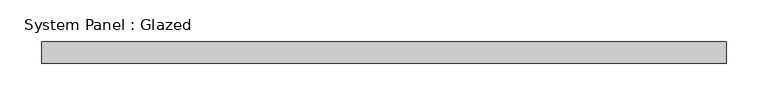
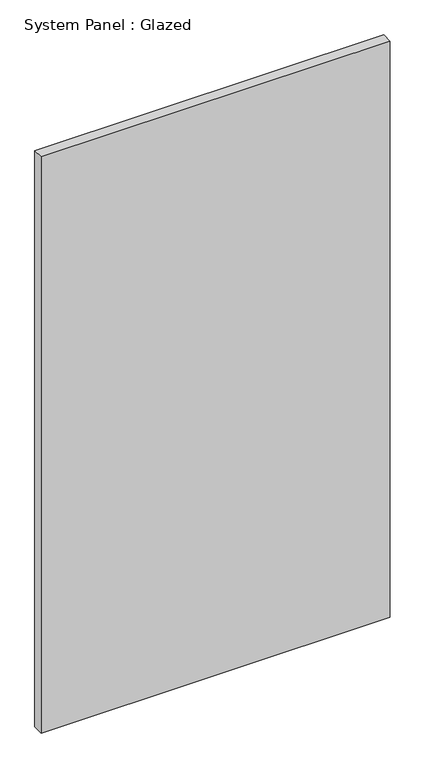
"""IFC4 building model written with IfcOpenShell, lengths in millimetres: plate geometry, System Panel : Glazed."""

from ifc_helpers import new_model, si_unit, origin, origin_with_axes, place, context, project, spatial, polyline, outline, extrude, source, transform, mapped, element, save


def system_panel_glazed_d26374ee(model_context):
    return source(origin(), model_context, "Body", "SweptSolid", [
        extrude(outline(polyline([(409.575, 19.05), (-409.575, 19.05), (-409.575, 44.45), (409.575, 44.45), (409.575, 19.05)])), origin_with_axes(), (0.0, 0.0, 1.0), 1428.75),
    ])


if __name__ == "__main__":
    model = new_model("IFC4")
    model_context = context("Model", 3, world=origin())
    ifc_project = project(units=[si_unit("LENGTHUNIT", "METRE", prefix="MILLI")], contexts=[model_context])
    site = spatial("IfcSite", under=ifc_project)
    building = spatial("IfcBuilding", under=site)
    placement = place(None, origin())
    system_panel_glazed_shape = system_panel_glazed_d26374ee(model_context)
    element("IfcPlate", 1, ObjectType="System Panel : Glazed", at=placement, inside=building, context=model_context, shape_type="MappedRepresentation", body=[
        mapped(system_panel_glazed_shape, transform((0.0, 0.0, 0.0), x_axis=(1.0, 0.0, 0.0), y_axis=(0.0, 1.0, 0.0), z_axis=(0.0, 0.0, 1.0))),
    ])
    save(model, "model.ifc")

# Revit data of these elements
# Type "System Panel : Glazed"
#   Construction Type Id = "GSP4R"
#   Analytic Construction = "1/8 in Pilkington single glazing"
#   Visual Light Transmittance = 0.9
#   Solar Heat Gain Coefficient = 0.86
#   Heat Transfer Coefficient (U) = 1.18115 BTU/(h·ft²·°F)
#   Define Thermal Properties by = 1
# Element 1 (IfcPlate, "System Panel : Glazed")
#   Materials on its faces: "Glass"
# Materials
#   "Glass": class "Glass", colour RGB 0 128 192, transparency 0.75, Description = "Soda Lime Glass", Cost = 0
